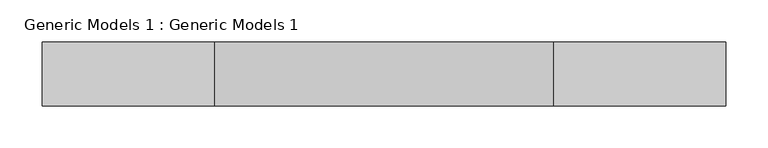
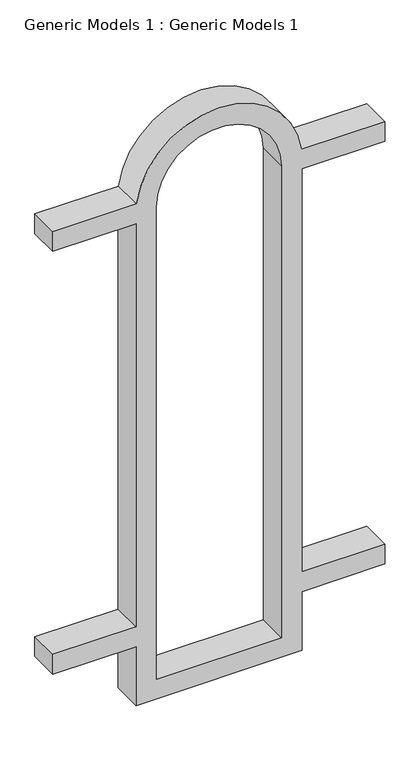
"""IFC4 building model written with IfcOpenShell, lengths in millimetres: proxy geometry, Generic Models 1 : Generic Models 1."""

from ifc_helpers import new_model, si_unit, point, frame, frame_2d, origin, place, context, project, spatial, polyline, circle_curve, trimmed, segment, composite_curve, outline, extrude, source, transform, mapped, element, save


def generic_models_1_generic_models_1_e4eb0336(model_context):
    return source(origin(), model_context, "Body", "SweptSolid", [
        extrude(outline(composite_curve([segment(polyline([(4851.4, -7057.8887575), (4851.4, -7262.6825076), (4800.6, -7262.6825076), (4800.6, -7059.4825076), (3759.2, -7059.4825076), (3759.2, -7262.6825076), (3708.4, -7262.6825076), (3708.4, -7059.4825076), (3556.0, -7059.4825076), (3556.0, -6653.0825076), (3708.4, -6653.0825076), (3708.4, -6449.8825076), (3759.2, -6449.8825076), (3759.2, -6653.0825076), (4800.6, -6653.0825076), (4800.6, -6449.8825076), (4851.4, -6449.8825076), (4851.4, -6654.6762577)]), True, "CONTINUOUS"), segment(trimmed(circle_curve(frame_2d((4826.0, -6856.2825076)), 203.2), [point((4851.4, -6654.6762577))], [point((4851.4, -7057.8887575))], False, "CARTESIAN"), True, "CONTINUOUS")], self_intersect=False), holes=[composite_curve([segment(trimmed(circle_curve(frame_2d((4826.0, -6856.2825076)), 152.4), [point((4826.0, -7008.6825076))], [point((4826.0, -6703.8825076))], True, "CARTESIAN"), True, "CONTINUOUS"), segment(polyline([(4826.0, -6703.8825076), (3606.8, -6703.8825076), (3606.8, -7008.6825076), (4826.0, -7008.6825076)]), True, "CONTINUOUS")], self_intersect=False)]), frame((0.0, -4810.2608295, 0.0), z_axis=(0.0, 1.0, 0.0), x_axis=(0.0, 0.0, 1.0)), (0.0, 0.0, 1.0), 76.2),
    ])


if __name__ == "__main__":
    model = new_model("IFC4")
    model_context = context("Model", 3, world=origin())
    ifc_project = project(units=[si_unit("LENGTHUNIT", "METRE", prefix="MILLI")], contexts=[model_context])
    site = spatial("IfcSite", under=ifc_project)
    building = spatial("IfcBuilding", under=site)
    placement = place(None, origin())
    generic_models_1_generic_models_1_shape = generic_models_1_generic_models_1_e4eb0336(model_context)
    element("IfcBuildingElementProxy", 1, Name="Generic Models 1 : Generic Models 1", ObjectType="Generic Models 1 : Generic Models 1", at=placement, inside=building, context=model_context, shape_type="MappedRepresentation", body=[
        mapped(generic_models_1_generic_models_1_shape, transform((0.0, 0.0, 0.0), x_axis=(1.0, 0.0, 0.0), y_axis=(0.0, 1.0, 0.0), z_axis=(0.0, 0.0, 1.0))),
    ])
    save(model, "model.ifc")

# Revit data of these elements
# Element 1 (IfcBuildingElementProxy, "Generic Models 1 : Generic Models 1")
#   Materials on its faces: "Aluminum"
# Materials
#   "Aluminum": class "Metal", colour RGB 244 245 246, transparency 0, Description = "Aluminum 6061", Cost = 0
